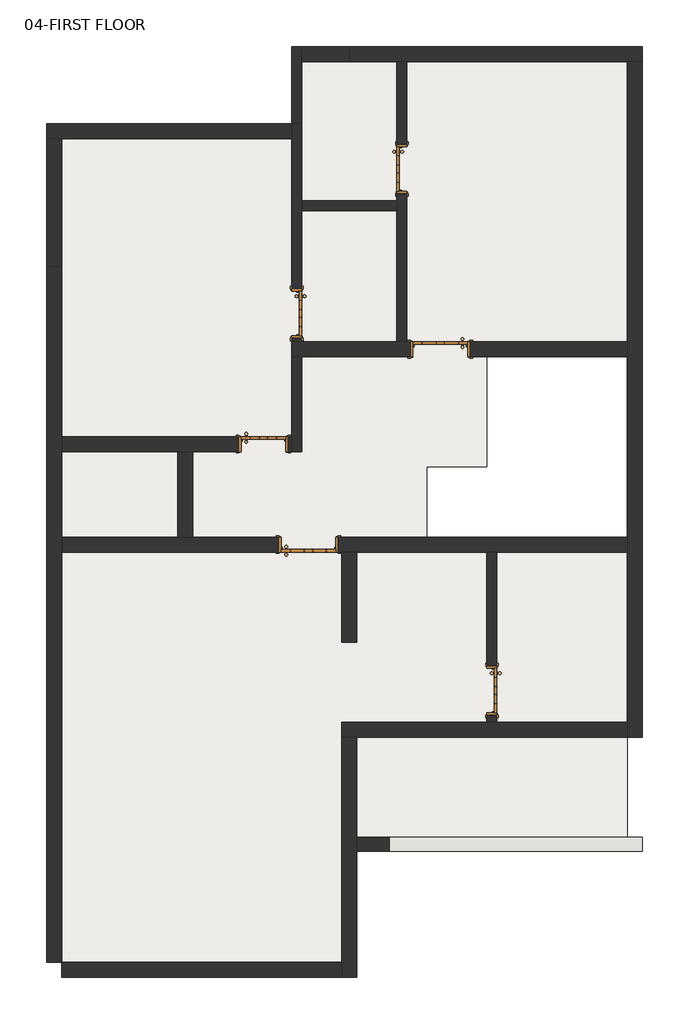
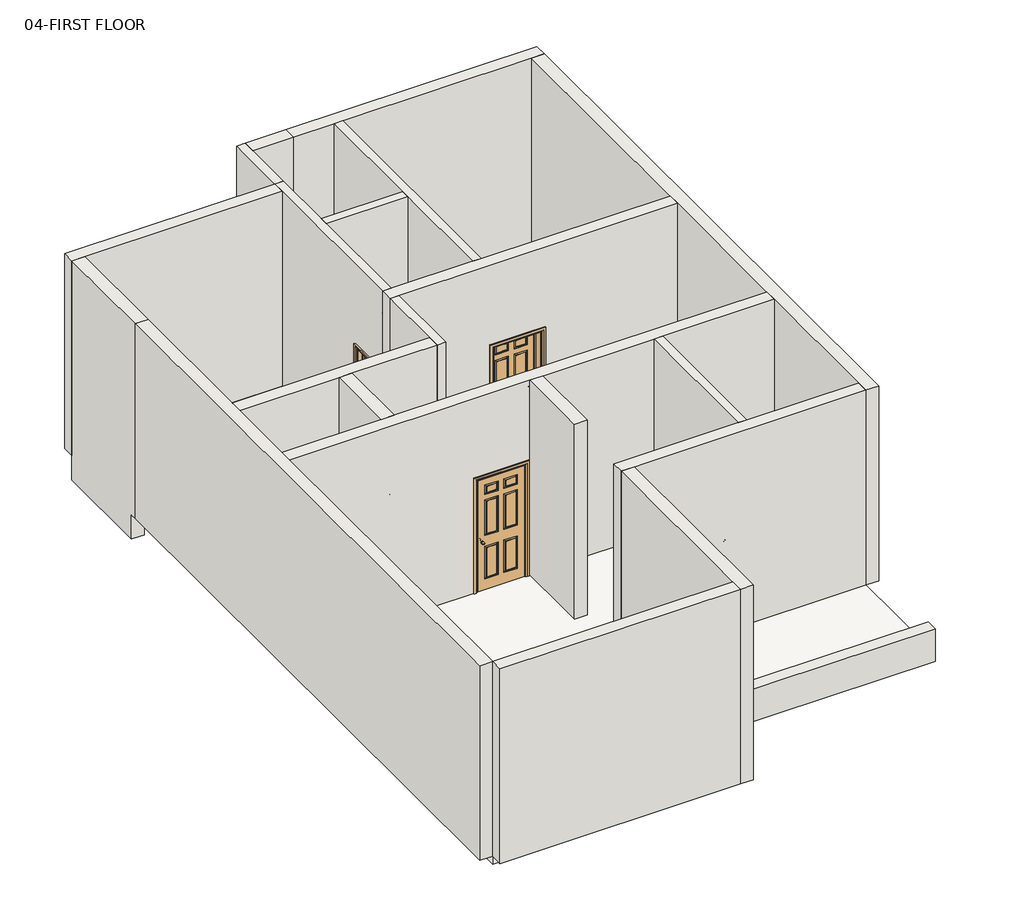
# One storey: 22 walls, 6 doors, 1 slab.
"""IFC4 building model written with IfcOpenShell, lengths in millimetres."""

from ifc_helpers import new_model, si_unit, frame, origin, place, context, project, spatial, polyline, outline, extrude, faceted_brep, transform, mapped, element, save
from components import intsgl_9_d1_bc548916, intsgl_9_d2_a593ccd7, intsgl_9_d2_8283ee4d, intsgl_9_d2_5357b631

model = new_model("IFC4")

# Units and contexts
model_context = context("Model", 3, world=origin())
ifc_project = project(units=[si_unit("LENGTHUNIT", "METRE", prefix="MILLI")], contexts=[model_context])

# Site, building, storey
site = spatial("IfcSite", under=ifc_project)
building = spatial("IfcBuilding", under=site)
storey = spatial("IfcBuildingStorey", under=building, Name="04-FIRST FLOOR", Elevation=3750.0)

# Doors
placement = place(None, origin())
intsgl_9_d1_shape = intsgl_9_d1_bc548916(model_context)
element("IfcDoor", 1, ObjectType="IntSgl (9) : D1", at=placement, inside=storey, context=model_context, shape_type="MappedRepresentation", body=[
    mapped(intsgl_9_d1_shape, transform((-10642.6792561, 410.7802318, 3750.0), x_axis=(1.0, 0.0, 0.0), y_axis=(0.0, 1.0, 0.0), z_axis=(0.0, 0.0, 1.0))),
])
element("IfcDoor", 2, ObjectType="IntSgl (9) : D1", at=placement, inside=storey, context=model_context, shape_type="MappedRepresentation", body=[
    mapped(intsgl_9_d1_shape, transform((-8667.6792561, 3335.7802318, 3750.0), x_axis=(-1.0, 0.0, 0.0), y_axis=(0.0, -1.0, 0.0), z_axis=(0.0, 0.0, 1.0))),
])
intsgl_9_d2_shape = intsgl_9_d2_a593ccd7(model_context)
element("IfcDoor", 3, ObjectType="IntSgl (9) : D2", at=placement, inside=storey, context=model_context, shape_type="MappedRepresentation", body=[
    mapped(intsgl_9_d2_shape, transform((-9242.6792561, 6038.2802318, 3750.0), x_axis=(0.0, -1.0, 0.0), y_axis=(1.0, 0.0, 0.0), z_axis=(0.0, 0.0, 1.0))),
])
intsgl_9_d2_2_shape = intsgl_9_d2_8283ee4d(model_context)
element("IfcDoor", 4, ObjectType="IntSgl (9) : D2", at=placement, inside=storey, context=model_context, shape_type="MappedRepresentation", body=[
    mapped(intsgl_9_d2_2_shape, transform((-10817.6792561, 3873.2802318, 3750.0), x_axis=(0.0, -1.0, 0.0), y_axis=(1.0, 0.0, 0.0), z_axis=(0.0, 0.0, 1.0))),
])
element("IfcDoor", 5, ObjectType="IntSgl (9) : D2", at=placement, inside=storey, context=model_context, shape_type="MappedRepresentation", body=[
    mapped(intsgl_9_d2_2_shape, transform((-7892.6792561, -1776.7197682, 3750.0), x_axis=(0.0, -1.0, 0.0), y_axis=(1.0, 0.0, 0.0), z_axis=(0.0, 0.0, 1.0))),
])
intsgl_9_d2_3_shape = intsgl_9_d2_5357b631(model_context)
element("IfcDoor", 6, ObjectType="IntSgl (9) : D2", at=placement, inside=storey, context=model_context, shape_type="MappedRepresentation", body=[
    mapped(intsgl_9_d2_3_shape, transform((-11317.6792561, 1915.7802318, 3750.0), x_axis=(1.0, 0.0, 0.0), y_axis=(0.0, 1.0, 0.0), z_axis=(0.0, 0.0, 1.0))),
])

# Slab
element("IfcSlab", 7, ObjectType="01-floor", at=placement, inside=storey, context=model_context, shape_type="SweptSolid", body=[
    extrude(outline(polyline([(-10742.6792561, 6488.2802318), (-10742.6792561, 7648.2802318), (-5867.6792561, 7648.2802318), (-5867.6792561, 3448.2802318), (-7967.6792561, 3448.2802318), (-7967.6792561, 1572.8802318), (-8867.6792561, 1572.8802318), (-8867.6792561, 298.2802318), (-5867.6792561, 298.2802318), (-5867.6792561, -3976.7197682), (-10142.6792561, -3976.7197682), (-10142.6792561, -5851.7197682), (-14342.6792561, -5851.7197682), (-14342.6792561, 6488.2802318), (-10742.6792561, 6488.2802318)])), frame((0.0, 0.0, 3600.0), z_axis=(0.0, 0.0, 1.0), x_axis=(1.0, 0.0, 0.0)), (0.0, 0.0, 1.0), 150.0),
])

# Walls
element("IfcWall", 8, ObjectType="01-225 WALL", at=placement, inside=storey, context=model_context, shape_type="Brep", body=[
    faceted_brep([(-10142.6792561, -5851.7197682, 3750.0), (-14342.6792561, -5851.7197682, 3750.0), (-14342.6792561, -5851.7197682, 7350.0), (-10142.6792561, -5851.7197682, 7350.0), (-10142.6792561, -6076.7197682, 3750.0), (-10142.6792561, -6076.7197682, 7350.0), (-14342.6792561, -6076.7197682, 7350.0), (-14342.6792561, -6076.7197682, 3750.0), (-14342.6792561, -5964.2197682, 3750.0)], [[[0, 1, 2, 3]], [[4, 5, 6, 7]], [[1, 0, 4, 7, 8]], [[3, 2, 6, 5]], [[0, 3, 5, 4]], [[2, 1, 8, 7, 6]]]),
])
element("IfcWall", 9, ObjectType="01-225 WALL", at=placement, inside=storey, context=model_context, shape_type="Brep", body=[
    faceted_brep([(-14342.6792561, -5851.7197682, 3750.0), (-14342.6792561, 298.2802318, 3750.0), (-14342.6792561, 523.2802318, 3750.0), (-14342.6792561, 1803.2802318, 3750.0), (-14342.6792561, 2028.2802318, 3750.0), (-14342.6792561, 4575.7802318, 3750.0), (-14342.6792561, 4575.7802318, 7350.0), (-14342.6792561, 2028.2802318, 7350.0), (-14342.6792561, 1803.2802318, 7350.0), (-14342.6792561, 523.2802318, 7350.0), (-14342.6792561, 298.2802318, 7350.0), (-14342.6792561, -5851.7197682, 7350.0), (-14567.6792561, -5851.7197682, 3750.0), (-14567.6792561, -5851.7197682, 7350.0), (-14567.6792561, 4575.7802318, 7350.0), (-14567.6792561, 4575.7802318, 3750.0)], [[[0, 1, 2, 3, 4, 5, 6, 7, 8, 9, 10, 11]], [[12, 13, 14, 15]], [[5, 4, 3, 2, 1, 0, 12, 15]], [[6, 5, 15, 14]], [[11, 10, 9, 8, 7, 6, 14, 13]], [[0, 11, 13, 12]]]),
])
element("IfcWall", 10, ObjectType="01-225 WALL", at=placement, inside=storey, context=model_context, shape_type="SweptSolid", body=[
    extrude(outline(polyline([(3300.0, -10742.6792561), (3300.0, -10142.6792561), (3750.0, -10142.6792561), (3750.0, -10030.1792561), (7350.0, -10030.1792561), (7350.0, -10742.6792561), (3300.0, -10742.6792561)])), frame((0.0, 7648.2802318, 0.0), z_axis=(0.0, 1.0, 0.0), x_axis=(0.0, 0.0, 1.0)), (0.0, 0.0, 1.0), 225.0),
])
element("IfcWall", 11, ObjectType="01-225 WALL", at=placement, inside=storey, context=model_context, shape_type="Brep", body=[
    faceted_brep([(-5867.6792561, 7648.2802318, 3750.0), (-5867.6792561, 3448.2802318, 3750.0), (-5867.6792561, 3223.2802318, 3750.0), (-5867.6792561, 523.2802318, 3750.0), (-5867.6792561, 298.2802318, 3750.0), (-5867.6792561, -2251.7197682, 3750.0), (-5867.6792561, -2476.7197682, 3750.0), (-5867.6792561, -2476.7197682, 7350.0), (-5867.6792561, -2251.7197682, 7350.0), (-5867.6792561, 298.2802318, 7350.0), (-5867.6792561, 523.2802318, 7350.0), (-5867.6792561, 3223.2802318, 7350.0), (-5867.6792561, 3448.2802318, 7350.0), (-5867.6792561, 7648.2802318, 7350.0), (-5642.6792561, 7648.2802318, 3750.0), (-5642.6792561, 7648.2802318, 7350.0), (-5642.6792561, -2476.7197682, 7350.0), (-5642.6792561, -2476.7197682, 3750.0)], [[[0, 1, 2, 3, 4, 5, 6, 7, 8, 9, 10, 11, 12, 13]], [[14, 15, 16, 17]], [[6, 5, 4, 3, 2, 1, 0, 14, 17]], [[13, 12, 11, 10, 9, 8, 7, 16, 15]], [[0, 13, 15, 14]], [[7, 6, 17, 16]]]),
])
element("IfcWall", 12, ObjectType="01-225 WALL", at=placement, inside=storey, context=model_context, shape_type="Brep", body=[
    faceted_brep([(-10892.6792561, 3448.2802318, 7350.0), (-10742.6792561, 3448.2802318, 7350.0), (-9317.6792561, 3448.2802318, 7350.0), (-9167.6792561, 3448.2802318, 7350.0), (-5867.6792561, 3448.2802318, 7350.0), (-5867.6792561, 3448.2802318, 3750.0), (-8217.6792561, 3448.2802318, 3750.0), (-8217.6792561, 3448.2802318, 5850.0), (-9117.6792561, 3448.2802318, 5850.0), (-9117.6792561, 3448.2802318, 3750.0), (-9167.6792561, 3448.2802318, 3750.0), (-9317.6792561, 3448.2802318, 3750.0), (-10742.6792561, 3448.2802318, 3750.0), (-10892.6792561, 3448.2802318, 3750.0), (-5867.6792561, 3223.2802318, 7350.0), (-10742.6792561, 3223.2802318, 7350.0), (-10892.6792561, 3223.2802318, 7350.0), (-10892.6792561, 3223.2802318, 3750.0), (-10742.6792561, 3223.2802318, 3750.0), (-9117.6792561, 3223.2802318, 3750.0), (-9117.6792561, 3223.2802318, 5850.0), (-8217.6792561, 3223.2802318, 5850.0), (-8217.6792561, 3223.2802318, 3750.0), (-5867.6792561, 3223.2802318, 3750.0)], [[[0, 1, 2, 3, 4, 5, 6, 7, 8, 9, 10, 11, 12, 13]], [[14, 15, 16, 17, 18, 19, 20, 21, 22, 23]], [[5, 23, 22, 6]], [[17, 13, 12, 11, 10, 9, 19, 18]], [[4, 3, 2, 1, 0, 16, 15, 14]], [[5, 4, 14, 23]], [[0, 13, 17, 16]], [[8, 20, 19, 9]], [[20, 8, 7, 21]], [[21, 7, 6, 22]]]),
])
element("IfcWall", 13, ObjectType="01-225 WALL", at=placement, inside=storey, context=model_context, shape_type="Brep", body=[
    faceted_brep([(-5867.6792561, -2251.7197682, 3750.0), (-7817.6792561, -2251.7197682, 3750.0), (-7967.6792561, -2251.7197682, 3750.0), (-10142.6792561, -2251.7197682, 3750.0), (-10142.6792561, -2251.7197682, 7350.0), (-7967.6792561, -2251.7197682, 7350.0), (-7817.6792561, -2251.7197682, 7350.0), (-5867.6792561, -2251.7197682, 7350.0), (-5867.6792561, -2476.7197682, 3750.0), (-5867.6792561, -2476.7197682, 7350.0), (-9917.6792561, -2476.7197682, 7350.0), (-10142.6792561, -2476.7197682, 7350.0), (-10142.6792561, -2476.7197682, 3750.0), (-9917.6792561, -2476.7197682, 3750.0)], [[[0, 1, 2, 3, 4, 5, 6, 7]], [[8, 9, 10, 11, 12, 13]], [[3, 2, 1, 0, 8, 13, 12]], [[7, 6, 5, 4, 11, 10, 9]], [[0, 7, 9, 8]], [[4, 3, 12, 11]]]),
])
element("IfcWall", 14, ObjectType="01-225 WALL", at=placement, inside=storey, context=model_context, shape_type="Brep", body=[
    faceted_brep([(-14342.6792561, 523.2802318, 7350.0), (-12605.1792561, 523.2802318, 7350.0), (-12380.1792561, 523.2802318, 7350.0), (-5867.6792561, 523.2802318, 7350.0), (-5867.6792561, 523.2802318, 3750.0), (-10192.6792561, 523.2802318, 3750.0), (-10192.6792561, 523.2802318, 5850.0), (-11092.6792561, 523.2802318, 5850.0), (-11092.6792561, 523.2802318, 3750.0), (-12380.1792561, 523.2802318, 3750.0), (-12605.1792561, 523.2802318, 3750.0), (-14342.6792561, 523.2802318, 3750.0), (-5867.6792561, 298.2802318, 7350.0), (-7817.6792561, 298.2802318, 7350.0), (-7967.6792561, 298.2802318, 7350.0), (-9917.6792561, 298.2802318, 7350.0), (-10142.6792561, 298.2802318, 7350.0), (-14342.6792561, 298.2802318, 7350.0), (-14342.6792561, 298.2802318, 3750.0), (-11092.6792561, 298.2802318, 3750.0), (-11092.6792561, 298.2802318, 5850.0), (-10192.6792561, 298.2802318, 5850.0), (-10192.6792561, 298.2802318, 3750.0), (-10142.6792561, 298.2802318, 3750.0), (-9917.6792561, 298.2802318, 3750.0), (-7967.6792561, 298.2802318, 3750.0), (-7817.6792561, 298.2802318, 3750.0), (-5867.6792561, 298.2802318, 3750.0)], [[[0, 1, 2, 3, 4, 5, 6, 7, 8, 9, 10, 11]], [[12, 13, 14, 15, 16, 17, 18, 19, 20, 21, 22, 23, 24, 25, 26, 27]], [[4, 27, 26, 25, 24, 23, 22, 5]], [[18, 11, 10, 9, 8, 19]], [[3, 2, 1, 0, 17, 16, 15, 14, 13, 12]], [[0, 11, 18, 17]], [[4, 3, 12, 27]], [[21, 6, 5, 22]], [[6, 21, 20, 7]], [[7, 20, 19, 8]]]),
])
element("IfcWall", 15, ObjectType="01-225 WALL", at=placement, inside=storey, context=model_context, shape_type="Brep", body=[
    faceted_brep([(-10892.6792561, 6713.2802318, 3750.0), (-14567.6792561, 6713.2802318, 3750.0), (-14567.6792561, 6713.2802318, 7350.0), (-10892.6792561, 6713.2802318, 7350.0), (-10892.6792561, 6488.2802318, 3750.0), (-10892.6792561, 6488.2802318, 7350.0), (-14342.6792561, 6488.2802318, 7350.0), (-14567.6792561, 6488.2802318, 7350.0), (-14567.6792561, 6488.2802318, 3750.0)], [[[0, 1, 2, 3]], [[4, 5, 6, 7, 8]], [[1, 0, 4, 8]], [[3, 2, 7, 6, 5]], [[2, 1, 8, 7]], [[0, 3, 5, 4]]]),
])
element("IfcWall", 16, ObjectType="01-225 WALL", at=placement, inside=storey, context=model_context, shape_type="Brep", body=[
    faceted_brep([(-14567.6792561, 6488.2802318, 3300.0), (-14567.6792561, 4688.2802318, 3300.0), (-14567.6792561, 4688.2802318, 3750.0), (-14567.6792561, 4575.7802318, 3750.0), (-14567.6792561, 4575.7802318, 7350.0), (-14567.6792561, 6488.2802318, 7350.0), (-14567.6792561, 6488.2802318, 3750.0), (-14342.6792561, 6488.2802318, 3300.0), (-14342.6792561, 6488.2802318, 7350.0), (-14342.6792561, 4575.7802318, 7350.0), (-14342.6792561, 4575.7802318, 3750.0), (-14342.6792561, 4688.2802318, 3750.0), (-14342.6792561, 4688.2802318, 3300.0)], [[[0, 1, 2, 3, 4, 5, 6]], [[7, 8, 9, 10, 11, 12]], [[1, 0, 7, 12]], [[5, 4, 9, 8]], [[4, 3, 10, 9]], [[10, 3, 2, 11]], [[2, 1, 12, 11]], [[0, 6, 5, 8, 7]]]),
])
element("IfcWall", 17, ObjectType="01-225 WALL", at=placement, inside=storey, context=model_context, shape_type="Brep", body=[
    faceted_brep([(-14342.6792561, 2028.2802318, 7350.0), (-10892.6792561, 2028.2802318, 7350.0), (-10892.6792561, 2028.2802318, 3750.0), (-10942.6792561, 2028.2802318, 3750.0), (-10942.6792561, 2028.2802318, 5850.0), (-11692.6792561, 2028.2802318, 5850.0), (-11692.6792561, 2028.2802318, 3750.0), (-14342.6792561, 2028.2802318, 3750.0), (-10892.6792561, 1803.2802318, 7350.0), (-12380.1792561, 1803.2802318, 7350.0), (-12605.1792561, 1803.2802318, 7350.0), (-14342.6792561, 1803.2802318, 7350.0), (-14342.6792561, 1803.2802318, 3750.0), (-12605.1792561, 1803.2802318, 3750.0), (-12380.1792561, 1803.2802318, 3750.0), (-11692.6792561, 1803.2802318, 3750.0), (-11692.6792561, 1803.2802318, 5850.0), (-10942.6792561, 1803.2802318, 5850.0), (-10942.6792561, 1803.2802318, 3750.0), (-10892.6792561, 1803.2802318, 3750.0)], [[[0, 1, 2, 3, 4, 5, 6, 7]], [[8, 9, 10, 11, 12, 13, 14, 15, 16, 17, 18, 19]], [[12, 7, 6, 15, 14, 13]], [[2, 19, 18, 3]], [[1, 0, 11, 10, 9, 8]], [[0, 7, 12, 11]], [[2, 1, 8, 19]], [[17, 4, 3, 18]], [[4, 17, 16, 5]], [[5, 16, 15, 6]]]),
])
element("IfcWall", 18, ObjectType="01-225 WALL", at=placement, inside=storey, context=model_context, shape_type="Brep", body=[
    faceted_brep([(-10030.1792561, 7648.2802318, 3750.0), (-9317.6792561, 7648.2802318, 3750.0), (-9167.6792561, 7648.2802318, 3750.0), (-5867.6792561, 7648.2802318, 3750.0), (-5642.6792561, 7648.2802318, 3750.0), (-5642.6792561, 7648.2802318, 7350.0), (-5867.6792561, 7648.2802318, 7350.0), (-9167.6792561, 7648.2802318, 7350.0), (-9317.6792561, 7648.2802318, 7350.0), (-10030.1792561, 7648.2802318, 7350.0), (-10030.1792561, 7873.2802318, 3750.0), (-10030.1792561, 7873.2802318, 7350.0), (-5642.6792561, 7873.2802318, 7350.0), (-5642.6792561, 7873.2802318, 3750.0), (-5867.6792561, 7873.2802318, 3750.0)], [[[0, 1, 2, 3, 4, 5, 6, 7, 8, 9]], [[10, 11, 12, 13, 14]], [[4, 3, 2, 1, 0, 10, 14, 13]], [[9, 8, 7, 6, 5, 12, 11]], [[0, 9, 11, 10]], [[5, 4, 13, 12]]]),
])
element("IfcWall", 19, ObjectType="01-225 WALL", at=placement, inside=storey, context=model_context, shape_type="SweptSolid", body=[
    extrude(outline(polyline([(-10142.6792561, -1051.7197682), (-10142.6792561, 298.2802318), (-9917.6792561, 298.2802318), (-9917.6792561, -1051.7197682), (-10142.6792561, -1051.7197682)])), frame((0.0, 0.0, 3750.0), z_axis=(0.0, 0.0, 1.0), x_axis=(1.0, 0.0, 0.0)), (0.0, 0.0, 1.0), 3600.0),
])
element("IfcWall", 20, ObjectType="01-225 WALL", at=placement, inside=storey, context=model_context, shape_type="SweptSolid", body=[
    extrude(outline(polyline([(-12605.1792561, 523.2802318), (-12605.1792561, 1803.2802318), (-12380.1792561, 1803.2802318), (-12380.1792561, 523.2802318), (-12605.1792561, 523.2802318)])), frame((0.0, 0.0, 3750.0), z_axis=(0.0, 0.0, 1.0), x_axis=(1.0, 0.0, 0.0)), (0.0, 0.0, 1.0), 3600.0),
])
element("IfcWall", 21, ObjectType="01-225 WALL", at=placement, inside=storey, context=model_context, shape_type="Brep", body=[
    faceted_brep([(-10142.6792561, -2476.7197682, 3750.0), (-10142.6792561, -5851.7197682, 3750.0), (-10142.6792561, -6076.7197682, 3750.0), (-10142.6792561, -6076.7197682, 7350.0), (-10142.6792561, -5851.7197682, 7350.0), (-10142.6792561, -2476.7197682, 7350.0), (-9917.6792561, -2476.7197682, 3750.0), (-9917.6792561, -2476.7197682, 7350.0), (-9917.6792561, -6076.7197682, 7350.0), (-9917.6792561, -6076.7197682, 3750.0)], [[[0, 1, 2, 3, 4, 5]], [[6, 7, 8, 9]], [[2, 1, 0, 6, 9]], [[5, 4, 3, 8, 7]], [[3, 2, 9, 8]], [[0, 5, 7, 6]]]),
])
element("IfcWall", 22, ObjectType="01-225 WALL MAIN", at=placement, inside=storey, context=model_context, shape_type="Brep", body=[
    faceted_brep([(-9917.6792561, -4186.7197682, 6450.0), (-9917.6792561, -4186.7197682, 3300.0), (-9430.1792561, -4186.7197682, 3300.0), (-9430.1792561, -4186.7197682, 3900.0), (-9430.1792561, -4186.7197682, 5850.0), (-9430.1792561, -4186.7197682, 6450.0), (-9917.6792561, -3976.7197682, 3300.0), (-9917.6792561, -3976.7197682, 6450.0), (-9430.1792561, -3976.7197682, 6450.0), (-9430.1792561, -3976.7197682, 5850.0), (-9430.1792561, -3976.7197682, 3900.0), (-9430.1792561, -3976.7197682, 3300.0)], [[[0, 1, 2, 3, 4, 5]], [[6, 7, 8, 9, 10, 11]], [[2, 1, 6, 11]], [[0, 5, 8, 7]], [[0, 7, 6, 1]], [[2, 11, 10, 9, 8, 5, 4, 3]]]),
])
element("IfcWall", 23, ObjectType="01-225 WALL MAIN", at=placement, inside=storey, context=model_context, shape_type="SweptSolid", body=[
    extrude(outline(polyline([(-5642.6792561, -4186.7197682), (-9430.1792561, -4186.7197682), (-9430.1792561, -3976.7197682), (-5642.6792561, -3976.7197682), (-5642.6792561, -4186.7197682)])), frame((0.0, 0.0, 3300.0), z_axis=(0.0, 0.0, 1.0), x_axis=(1.0, 0.0, 0.0)), (0.0, 0.0, 1.0), 600.0),
])
element("IfcWall", 24, ObjectType="02-150 WALL", at=placement, inside=storey, context=model_context, shape_type="Brep", body=[
    faceted_brep([(-10892.6792561, 3223.2802318, 3750.0), (-10892.6792561, 2028.2802318, 3750.0), (-10892.6792561, 1803.2802318, 3750.0), (-10892.6792561, 1803.2802318, 7350.0), (-10892.6792561, 2028.2802318, 7350.0), (-10892.6792561, 3223.2802318, 7350.0), (-10742.6792561, 3223.2802318, 3750.0), (-10742.6792561, 3223.2802318, 7350.0), (-10742.6792561, 1803.2802318, 7350.0), (-10742.6792561, 1803.2802318, 3750.0)], [[[0, 1, 2, 3, 4, 5]], [[6, 7, 8, 9]], [[2, 1, 0, 6, 9]], [[5, 4, 3, 8, 7]], [[0, 5, 7, 6]], [[3, 2, 9, 8]]]),
])
element("IfcWall", 25, ObjectType="02-150 WALL", at=placement, inside=storey, context=model_context, shape_type="Brep", body=[
    faceted_brep([(-10892.6792561, 3448.2802318, 7350.0), (-10892.6792561, 6488.2802318, 7350.0), (-10892.6792561, 6713.2802318, 7350.0), (-10892.6792561, 6713.2802318, 3750.0), (-10892.6792561, 6488.2802318, 3750.0), (-10892.6792561, 4248.2802318, 3750.0), (-10892.6792561, 4248.2802318, 5850.0), (-10892.6792561, 3498.2802318, 5850.0), (-10892.6792561, 3498.2802318, 3750.0), (-10892.6792561, 3448.2802318, 3750.0), (-10742.6792561, 6713.2802318, 7350.0), (-10742.6792561, 5563.2802318, 7350.0), (-10742.6792561, 5413.2802318, 7350.0), (-10742.6792561, 3448.2802318, 7350.0), (-10742.6792561, 3448.2802318, 3750.0), (-10742.6792561, 3498.2802318, 3750.0), (-10742.6792561, 3498.2802318, 5850.0), (-10742.6792561, 4248.2802318, 5850.0), (-10742.6792561, 4248.2802318, 3750.0), (-10742.6792561, 5413.2802318, 3750.0), (-10742.6792561, 5563.2802318, 3750.0), (-10742.6792561, 6713.2802318, 3750.0)], [[[0, 1, 2, 3, 4, 5, 6, 7, 8, 9]], [[10, 11, 12, 13, 14, 15, 16, 17, 18, 19, 20, 21]], [[14, 9, 8, 15]], [[3, 21, 20, 19, 18, 5, 4]], [[2, 1, 0, 13, 12, 11, 10]], [[0, 9, 14, 13]], [[3, 2, 10, 21]], [[7, 16, 15, 8]], [[16, 7, 6, 17]], [[17, 6, 5, 18]]]),
])
element("IfcWall", 26, ObjectType="02-150 WALL", at=placement, inside=storey, context=model_context, shape_type="Brep", body=[
    faceted_brep([(-9317.6792561, 3448.2802318, 7350.0), (-9317.6792561, 5413.2802318, 7350.0), (-9317.6792561, 5563.2802318, 7350.0), (-9317.6792561, 7648.2802318, 7350.0), (-9317.6792561, 7648.2802318, 3750.0), (-9317.6792561, 6413.2802318, 3750.0), (-9317.6792561, 6413.2802318, 5850.0), (-9317.6792561, 5663.2802318, 5850.0), (-9317.6792561, 5663.2802318, 3750.0), (-9317.6792561, 5563.2802318, 3750.0), (-9317.6792561, 5413.2802318, 3750.0), (-9317.6792561, 3448.2802318, 3750.0), (-9167.6792561, 7648.2802318, 7350.0), (-9167.6792561, 3448.2802318, 7350.0), (-9167.6792561, 3448.2802318, 3750.0), (-9167.6792561, 5663.2802318, 3750.0), (-9167.6792561, 5663.2802318, 5850.0), (-9167.6792561, 6413.2802318, 5850.0), (-9167.6792561, 6413.2802318, 3750.0), (-9167.6792561, 7648.2802318, 3750.0)], [[[0, 1, 2, 3, 4, 5, 6, 7, 8, 9, 10, 11]], [[12, 13, 14, 15, 16, 17, 18, 19]], [[4, 19, 18, 5]], [[14, 11, 10, 9, 8, 15]], [[3, 2, 1, 0, 13, 12]], [[4, 3, 12, 19]], [[0, 11, 14, 13]], [[7, 16, 15, 8]], [[16, 7, 6, 17]], [[17, 6, 5, 18]]]),
])
element("IfcWall", 27, ObjectType="02-150 WALL", at=placement, inside=storey, context=model_context, shape_type="Brep", body=[
    faceted_brep([(-10742.6792561, 6713.2802318, 3300.0), (-10742.6792561, 7648.2802318, 3300.0), (-10742.6792561, 7873.2802318, 3300.0), (-10742.6792561, 7873.2802318, 7350.0), (-10742.6792561, 7648.2802318, 7350.0), (-10742.6792561, 6713.2802318, 7350.0), (-10742.6792561, 6713.2802318, 3750.0), (-10892.6792561, 6713.2802318, 3300.0), (-10892.6792561, 6713.2802318, 3750.0), (-10892.6792561, 6713.2802318, 7350.0), (-10892.6792561, 7873.2802318, 7350.0), (-10892.6792561, 7873.2802318, 3300.0)], [[[0, 1, 2, 3, 4, 5, 6]], [[7, 8, 9, 10, 11]], [[2, 1, 0, 7, 11]], [[5, 4, 3, 10, 9]], [[3, 2, 11, 10]], [[0, 6, 5, 9, 8, 7]]]),
])
element("IfcWall", 28, ObjectType="02-150 WALL", at=placement, inside=storey, context=model_context, shape_type="SweptSolid", body=[
    extrude(outline(polyline([(-9317.6792561, 5413.2802318), (-10742.6792561, 5413.2802318), (-10742.6792561, 5563.2802318), (-9317.6792561, 5563.2802318), (-9317.6792561, 5413.2802318)])), frame((0.0, 0.0, 3750.0), z_axis=(0.0, 0.0, 1.0), x_axis=(1.0, 0.0, 0.0)), (0.0, 0.0, 1.0), 3600.0),
])
element("IfcWall", 29, ObjectType="02-150 WALL", at=placement, inside=storey, context=model_context, shape_type="SweptSolid", body=[
    extrude(outline(polyline([(-2251.7197682, 7350.0), (298.2802318, 7350.0), (298.2802318, 3750.0), (-1401.7197682, 3750.0), (-1401.7197682, 5850.0), (-2151.7197682, 5850.0), (-2151.7197682, 3750.0), (-2251.7197682, 3750.0), (-2251.7197682, 7350.0)])), frame((-7967.6792561, 0.0, 0.0), z_axis=(1.0, 0.0, 0.0), x_axis=(0.0, 1.0, 0.0)), (0.0, 0.0, 1.0), 150.0),
])

save(model, "model.ifc")

# Revit data of these elements
# Type "IntSgl (9) : D1"
#   Type Mark = "46"
#   Operation = "SingleSwingRight"
#   Manufacturer = "Revit"
#   Keynote = "L20"
#   UnderCut = 8 mm
#   Tolerance = 2 mm
#   Thickness = 38 mm
#   Structural Tolerance = 8 mm
#   StopDepth = 32 mm
#   Stop Thickness = 19 mm
#   Stile Top Rail = 125 mm
#   Stile Shutting = 125 mm
#   Stile Muntin Rail = 100 mm
#   Stile Lock Rail = 200 mm
#   Stile Intermediate/Frieze = 100 mm
#   Stile Hanging = 125 mm
#   Stile Bottom Rail = 200 mm
#   Rough Width = 900 mm
#   Rough Height = 2100 mm
#   Height to Top Lock Rail = 1000 mm
#   Handle Z Distance = 900 mm
#   Handle X Distance = 75 mm
#   Frame Thickness = 32 mm
#   Door Panel Width = 816 mm
#   Height = 2100 mm
#   Width = 900 mm
#   Door Panel Thickness = 38 mm
#   Door Panel Offset = 0 mm
#   Door Panel Height = 2050 mm
#   Architrave Setback = 5 mm
#   Vis - Ironmongery = yes
#   Material Ironmongery = Door - Handle
#   Material Frame = Door - Frame/Mullion
#   Material Door = Door - Panel
#   Material Architrave = Door - Architrave
#   Function = (empty or 0)
#   Wall Closure = (empty or 0)
# Type "IntSgl (9) : D2"
#   Type Mark = "50"
#   Operation = "SingleSwingRight"
#   Manufacturer = "Revit"
#   Keynote = "L20"
#   UnderCut = 8 mm
#   Tolerance = 2 mm
#   Thickness = 38 mm
#   Structural Tolerance = 8 mm
#   StopDepth = 32 mm
#   Stop Thickness = 19 mm
#   Stile Top Rail = 125 mm
#   Stile Shutting = 125 mm
#   Stile Muntin Rail = 100 mm
#   Stile Lock Rail = 200 mm
#   Stile Intermediate/Frieze = 100 mm
#   Stile Hanging = 125 mm
#   Stile Bottom Rail = 200 mm
#   Rough Width = 750 mm
#   Rough Height = 2100 mm
#   Height to Top Lock Rail = 1000 mm
#   Handle Z Distance = 900 mm
#   Handle X Distance = 75 mm
#   Frame Thickness = 32 mm
#   Door Panel Width = 666 mm
#   Height = 2100 mm
#   Width = 750 mm
#   Door Panel Thickness = 38 mm
#   Door Panel Offset = 0 mm
#   Door Panel Height = 2050 mm
#   Architrave Setback = 5 mm
#   Vis - Ironmongery = yes
#   Material Ironmongery = Door - Handle
#   Material Frame = Door - Frame/Mullion
#   Material Door = Door - Panel
#   Material Architrave = Door - Architrave
#   Function = (empty or 0)
#   Wall Closure = (empty or 0)
# Type "01-floor"
#   Description = "Generic Floor (Material By Category), 12\" thick"
#   Assembly Code = "B1010"
#   Type Mark = "G01"
#   Function = 0
#   Layers, outside or top first: 150 mm no material (function 1)
# Type "01-225 WALL"
#   Description = "Generic Wall (Material By Category), 200mm thick"
#   Assembly Code = "B2010"
#   Type Mark = "G06"
#   Layers, outside or top first: 225 mm no material (function 1)
# Type "01-225 WALL MAIN"
#   Description = "Generic Wall (Material By Category), 200mm thick"
#   Assembly Code = "B2010"
#   Type Mark = "G06"
#   Layers, outside or top first: 5 mm "01-WHITE WALL PAINT" (function 4); 200 mm "01-DEFAULT WALL" (function 1); 5 mm "01-WHITE WALL PAINT" (function 5)
# Type "02-150 WALL"
#   Description = "Generic Wall (Material By Category), 200mm thick"
#   Assembly Code = "B2010"
#   Type Mark = "G06"
#   Layers, outside or top first: 150 mm no material (function 1)
# Elements 1, 2 (IfcDoor, "IntSgl (9) : D1")
#   Phase Created = New Construction
#   Materials on its faces: "Door - Panel", "Door - Architrave", "Door - Frame/Mullion", "Door - Handle"
# Elements 3, 4, 5, 6 (IfcDoor, "IntSgl (9) : D2")
#   Phase Created = New Construction
#   Materials on its faces: "Door - Panel", "Door - Architrave", "Door - Frame/Mullion", "Door - Handle"
# Element 7 (IfcSlab, "01-floor")
#   Height Offset From Level = 0 mm
#   Phase Created = New Construction
#   Materials on its faces: "Default Floor"
# Elements 8, 9, 11, 12, 13, 14, 15, 17, 18, 19, 20, 21 (IfcWall, "01-225 WALL")
#   Top Offset = 0 mm
#   Base Offset = 0 mm
#   wall height = 3600 mm
#   Phase Created = New Construction
#   Base Constraint = 04-FIRST FLOOR
#   Top Constraint = 07-ROOF LEVEL
#   Materials on its faces: "Default Wall"
# Elements 10, 16 (IfcWall, "01-225 WALL")
#   built-in parameter 1001111 = -450 mm
#   Top Offset = 0 mm
#   Base Offset = -450 mm
#   wall height = 4050 mm
#   Phase Created = New Construction
#   Base Constraint = 04-FIRST FLOOR
#   Top Constraint = 07-ROOF LEVEL
#   Materials on its faces: "Default Wall"
# Element 22 (IfcWall, "01-225 WALL MAIN")
#   built-in parameter 1001111 = -450 mm
#   Top Offset = -300 mm
#   Base Offset = -450 mm
#   wall height = 3150 mm
#   Phase Created = New Construction
#   Base Constraint = 04-FIRST FLOOR
#   Top Constraint = 06-CEILING
#   Materials on its faces: "Default Wall", "01-WHITE WALL PAINT"
# Element 23 (IfcWall, "01-225 WALL MAIN")
#   built-in parameter 1001111 = -450 mm
#   Top Offset = -1950 mm
#   Base Offset = -450 mm
#   wall height = 600 mm
#   Phase Created = New Construction
#   Base Constraint = 04-FIRST FLOOR
#   Top Constraint = 05-LINTEL 2
#   Materials on its faces: "Default Wall", "01-WHITE WALL PAINT"
# Elements 24, 25, 26, 28, 29 (IfcWall, "02-150 WALL")
#   Top Offset = 0 mm
#   Base Offset = 0 mm
#   wall height = 3600 mm
#   Phase Created = New Construction
#   Base Constraint = 04-FIRST FLOOR
#   Top Constraint = 07-ROOF LEVEL
#   Materials on its faces: "Default Wall"
# Element 27 (IfcWall, "02-150 WALL")
#   built-in parameter 1001111 = -450 mm
#   Top Offset = 0 mm
#   Base Offset = -450 mm
#   wall height = 4050 mm
#   Phase Created = New Construction
#   Base Constraint = 04-FIRST FLOOR
#   Top Constraint = 07-ROOF LEVEL
#   Materials on its faces: "Default Wall"
# Materials
#   "Door - Handle": colour RGB 247 247 247, transparency 0
#   "Door - Frame/Mullion": colour RGB 212 179 113, transparency 0
#   "Door - Panel": colour RGB 154 90 5, transparency 0
#   "Door - Architrave": colour RGB 154 90 5, transparency 0
#   "01-WHITE WALL PAINT": class "Generic", colour RGB 242 242 255, transparency 0, Description = "Acoustic Ceiling Tile 24 x 48", Cost = 0
#   "01-DEFAULT WALL": class "Generic", colour RGB 242 242 255, transparency 0, Description = "Acoustic Ceiling Tile 24 x 48", Cost = 0
#   "Default Floor": colour RGB 128 128 128, transparency 0, Cost = 0
#   "Default Wall": colour RGB 192 192 192, transparency 0, Cost = 0
